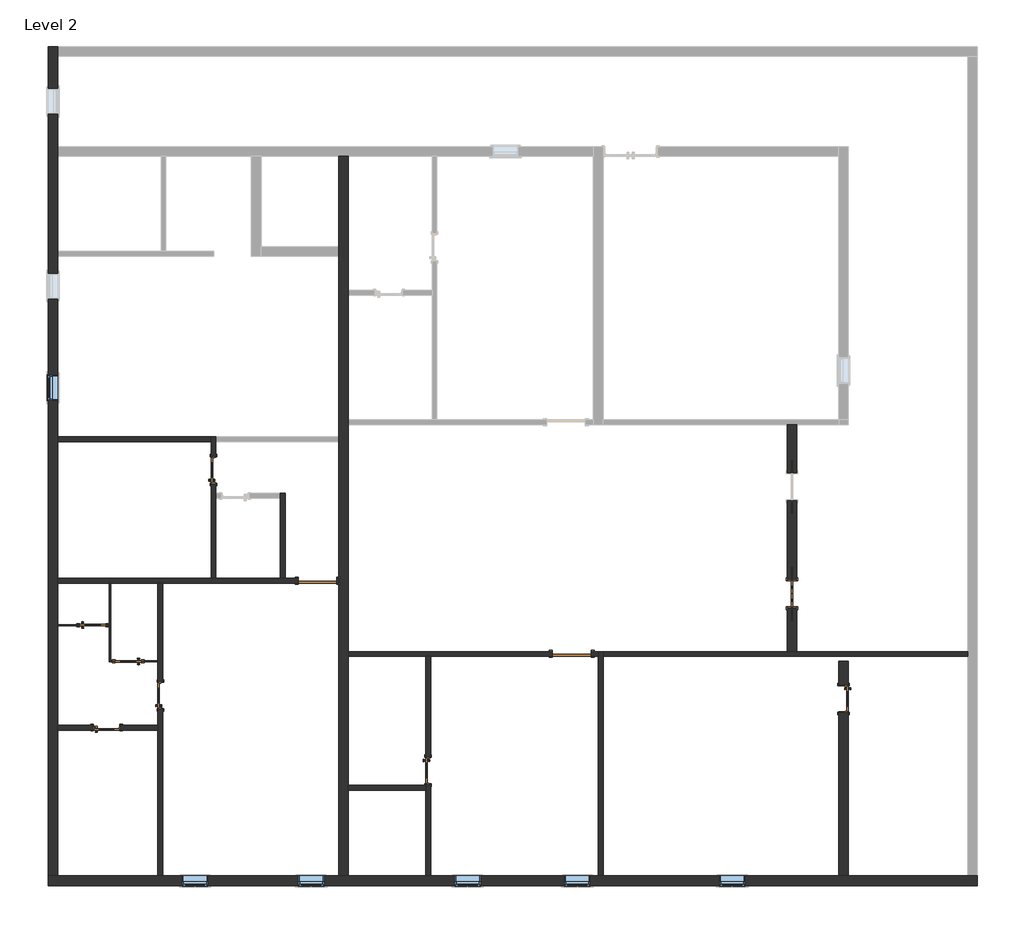
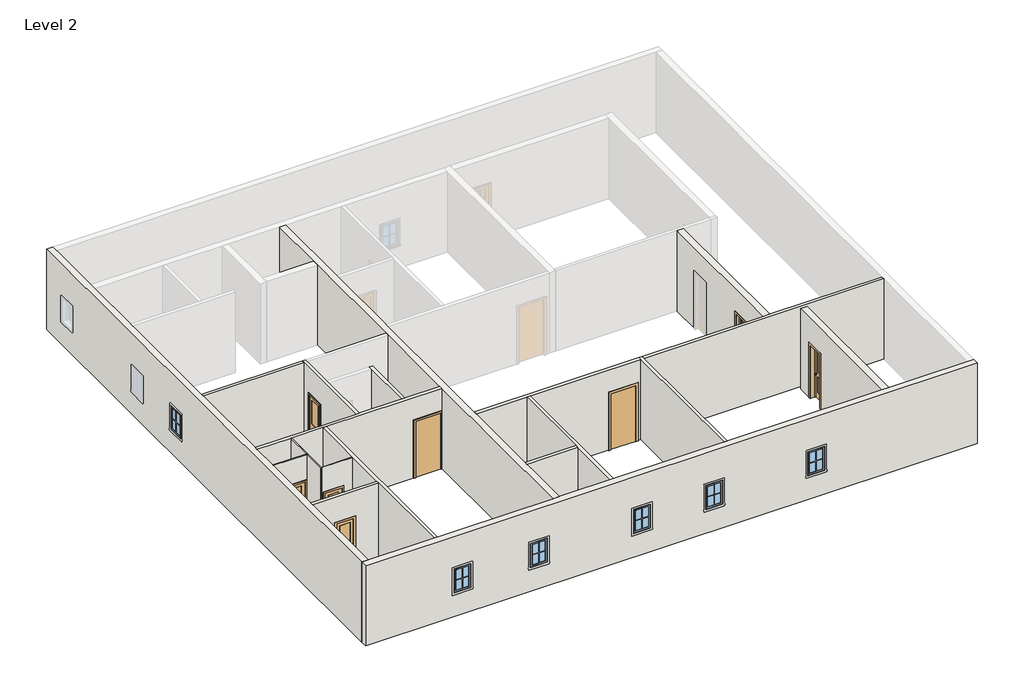
# One storey, part 1 of 2: 19 walls, 10 doors, 6 windows.
"""IFC4 building model written with IfcOpenShell, lengths in millimetres."""

from ifc_helpers import new_model, si_unit, frame, origin, place, context, project, spatial, polyline, outline, extrude, faceted_brep, transform, mapped, element, save
from components import door_interior_double_pocket_2_panel_wood_door_interior_52fbc1e8, door_interior_single_2_panel_wood_door_interior_single_2_03d66c98, door_interior_single_2_panel_wood_door_interior_single_2_a051e6ed, door_interior_single_2_panel_wood_door_interior_single_2_5f4e2ecc, door_interior_single_2_panel_wood_d3_c9a7c184, door_305aa2a5, window_bab9308a, window_25e7c868

model = new_model("IFC4")

# Units and contexts
model_context = context("Model", 3, world=origin())
ifc_project = project(units=[si_unit("LENGTHUNIT", "METRE", prefix="MILLI")], contexts=[model_context])

# Site, building, storey
site = spatial("IfcSite", under=ifc_project)
building = spatial("IfcBuilding", under=site)
storey = spatial("IfcBuildingStorey", under=building, Name="Level 2", Elevation=457.2)

# Doors
placement = place(None, origin())
door_interior_double_pocket_2_panel_wood_door_interior_shape = door_interior_double_pocket_2_panel_wood_door_interior_52fbc1e8(model_context)
element("IfcDoor", 1, ObjectType="Door-Interior-Double-Pocket-2_Panel-Wood : Door-Interior-Double-Pocket-2_Panel-Wood", at=placement, inside=storey, context=model_context, shape_type="MappedRepresentation", body=[
    mapped(door_interior_double_pocket_2_panel_wood_door_interior_shape, transform((5604.2549703, -2194.6409081, 457.2), x_axis=(0.0, -1.0, 0.0), y_axis=(1.0, 0.0, 0.0), z_axis=(0.0, 0.0, 1.0))),
])
door_interior_single_2_panel_wood_door_interior_single_2_shape = door_interior_single_2_panel_wood_door_interior_single_2_03d66c98(model_context)
element("IfcDoor", 2, ObjectType="Door-Interior-Single-2_Panel-Wood : Door-Interior-Single-2_Panel-Wood", at=placement, inside=storey, context=model_context, shape_type="MappedRepresentation", body=[
    mapped(door_interior_single_2_panel_wood_door_interior_single_2_shape, transform((-2989.8496667, -6372.9409081, 457.2), x_axis=(0.0, -1.0, 0.0), y_axis=(1.0, 0.0, 0.0), z_axis=(0.0, 0.0, 1.0))),
])
element("IfcDoor", 3, ObjectType="Door-Interior-Single-2_Panel-Wood : Door-Interior-Single-2_Panel-Wood", at=placement, inside=storey, context=model_context, shape_type="MappedRepresentation", body=[
    mapped(door_interior_single_2_panel_wood_door_interior_single_2_shape, transform((-10578.7200297, -5360.1159081, 457.2), x_axis=(1.0, 0.0, 0.0), y_axis=(0.0, 1.0, 0.0), z_axis=(0.0, 0.0, 1.0))),
])
door_interior_single_2_panel_wood_door_interior_single_2_2_shape = door_interior_single_2_panel_wood_door_interior_single_2_a051e6ed(model_context)
element("IfcDoor", 4, ObjectType="Door-Interior-Single-2_Panel-Wood : Door-Interior-Single-2_Panel-Wood", at=placement, inside=storey, context=model_context, shape_type="MappedRepresentation", body=[
    mapped(door_interior_single_2_panel_wood_door_interior_single_2_2_shape, transform((-9315.0700297, -4594.9409081, 457.2), x_axis=(0.0, 1.0, 0.0), y_axis=(-1.0, 0.0, 0.0), z_axis=(0.0, 0.0, 1.0))),
])
element("IfcDoor", 5, ObjectType="Door-Interior-Single-2_Panel-Wood : Door-Interior-Single-2_Panel-Wood", at=placement, inside=storey, context=model_context, shape_type="MappedRepresentation", body=[
    mapped(door_interior_single_2_panel_wood_door_interior_single_2_2_shape, transform((-8057.7700297, 726.3590919, 457.2), x_axis=(0.0, 1.0, 0.0), y_axis=(-1.0, 0.0, 0.0), z_axis=(0.0, 0.0, 1.0))),
])
door_interior_single_2_panel_wood_door_interior_single_2_3_shape = door_interior_single_2_panel_wood_door_interior_single_2_5f4e2ecc(model_context)
element("IfcDoor", 6, ObjectType="Door-Interior-Single-2_Panel-Wood : Door-Interior-Single-2_Panel-Wood", at=placement, inside=storey, context=model_context, shape_type="MappedRepresentation", body=[
    mapped(door_interior_single_2_panel_wood_door_interior_single_2_3_shape, transform((6826.6299703, -4677.4909081, 457.2), x_axis=(0.0, -1.0, 0.0), y_axis=(1.0, 0.0, 0.0), z_axis=(0.0, 0.0, 1.0))),
])
door_interior_single_2_panel_wood_d3_shape = door_interior_single_2_panel_wood_d3_c9a7c184(model_context)
element("IfcDoor", 7, ObjectType="Door-Interior-Single-2_Panel-Wood : d3", at=placement, inside=storey, context=model_context, shape_type="MappedRepresentation", body=[
    mapped(door_interior_single_2_panel_wood_d3_shape, transform((-10905.7021106, -2941.2913376, 457.2), x_axis=(1.0, 0.0, 0.0), y_axis=(0.0, 1.0, 0.0), z_axis=(0.0, 0.0, 1.0))),
])
element("IfcDoor", 8, ObjectType="Door-Interior-Single-2_Panel-Wood : d3", at=placement, inside=storey, context=model_context, shape_type="MappedRepresentation", body=[
    mapped(door_interior_single_2_panel_wood_d3_shape, transform((-10067.5021106, -3785.3159081, 457.2), x_axis=(-1.0, 0.0, 0.0), y_axis=(0.0, -1.0, 0.0), z_axis=(0.0, 0.0, 1.0))),
])
door_shape = door_305aa2a5(model_context)
element("IfcDoor", 9, ObjectType="Single-Flush : 36\" x 84\"", at=placement, inside=storey, context=model_context, shape_type="MappedRepresentation", body=[
    mapped(door_shape, transform((-5597.1450297, -1889.8409081, 457.2), x_axis=(1.0, 0.0, 0.0), y_axis=(0.0, 1.0, 0.0), z_axis=(0.0, 0.0, 1.0))),
])
element("IfcDoor", 10, ObjectType="Single-Flush : 36\" x 84\"", at=placement, inside=storey, context=model_context, shape_type="MappedRepresentation", body=[
    mapped(door_shape, transform((403.6049703, -3617.0409081, 457.2), x_axis=(1.0, 0.0, 0.0), y_axis=(0.0, 1.0, 0.0), z_axis=(0.0, 0.0, 1.0))),
])

# Walls
element("IfcWall", 11, ObjectType="1\"", at=placement, inside=storey, context=model_context, shape_type="SweptSolid", body=[
    extrude(outline(polyline([(3505.2, -10512.0021106), (3505.2, -11731.2450297), (457.2, -11731.2450297), (457.2, -11235.9021106), (2514.6, -11235.9021106), (2514.6, -10575.5021106), (457.2, -10575.5021106), (457.2, -10512.0021106), (3505.2, -10512.0021106)])), frame((0.0, -2950.8163376, 0.0), z_axis=(0.0, 1.0, 0.0), x_axis=(0.0, 0.0, 1.0)), (0.0, 0.0, 1.0), 25.4),
])
element("IfcWall", 12, ObjectType="1\"", at=placement, inside=storey, context=model_context, shape_type="Brep", body=[
    faceted_brep([(-10486.6021106, -3801.1909081, 457.2), (-10486.6021106, -3775.7909081, 457.2), (-10486.6021106, -1946.9909081, 457.2), (-10486.6021106, -1946.9909081, 3505.2), (-10486.6021106, -3775.7909081, 3505.2), (-10486.6021106, -3801.1909081, 3505.2), (-10512.0021106, -3801.1909081, 457.2), (-10512.0021106, -3801.1909081, 3505.2), (-10512.0021106, -2950.8163376, 3505.2), (-10512.0021106, -2925.4163376, 3505.2), (-10512.0021106, -1946.9909081, 3505.2), (-10512.0021106, -1946.9909081, 457.2), (-10512.0021106, -2925.4163376, 457.2), (-10512.0021106, -2950.8163376, 457.2)], [[[0, 1, 2, 3, 4, 5]], [[6, 7, 8, 9, 10, 11, 12, 13]], [[2, 1, 0, 6, 13, 12, 11]], [[5, 4, 3, 10, 9, 8, 7]], [[3, 2, 11, 10]], [[0, 5, 7, 6]]]),
])
element("IfcWall", 13, ObjectType="1\"", at=placement, inside=storey, context=model_context, shape_type="SweptSolid", body=[
    extrude(outline(polyline([(3505.2, -9369.0450297), (3505.2, -10486.6021106), (457.2, -10486.6021106), (457.2, -10397.7021106), (2514.6, -10397.7021106), (2514.6, -9737.3021106), (457.2, -9737.3021106), (457.2, -9369.0450297), (3505.2, -9369.0450297)])), frame((0.0, -3801.1909081, 0.0), z_axis=(0.0, 1.0, 0.0), x_axis=(0.0, 0.0, 1.0)), (0.0, 0.0, 1.0), 25.4),
])
element("IfcWall", 14, ObjectType="4.5\" wall", at=placement, inside=storey, context=model_context, shape_type="Brep", body=[
    faceted_brep([(-9254.7450297, -1946.9909081, 3505.2), (-9254.7450297, -8855.7909081, 3505.2), (-9254.7450297, -8855.7909081, 457.2), (-9254.7450297, -4925.1409081, 457.2), (-9254.7450297, -4925.1409081, 2514.6), (-9254.7450297, -4264.7409081, 2514.6), (-9254.7450297, -4264.7409081, 457.2), (-9254.7450297, -1946.9909081, 457.2), (-9369.0450297, -8855.7909081, 3505.2), (-9369.0450297, -5414.0909081, 3505.2), (-9369.0450297, -5299.7909081, 3505.2), (-9369.0450297, -3801.1909081, 3505.2), (-9369.0450297, -3775.7909081, 3505.2), (-9369.0450297, -1946.9909081, 3505.2), (-9369.0450297, -1946.9909081, 457.2), (-9369.0450297, -3775.7909081, 457.2), (-9369.0450297, -3801.1909081, 457.2), (-9369.0450297, -4264.7409081, 457.2), (-9369.0450297, -4264.7409081, 2514.6), (-9369.0450297, -4925.1409081, 2514.6), (-9369.0450297, -4925.1409081, 457.2), (-9369.0450297, -5299.7909081, 457.2), (-9369.0450297, -5414.0909081, 457.2), (-9369.0450297, -8855.7909081, 457.2)], [[[0, 1, 2, 3, 4, 5, 6, 7]], [[8, 9, 10, 11, 12, 13, 14, 15, 16, 17, 18, 19, 20, 21, 22, 23]], [[2, 23, 22, 21, 20, 3]], [[14, 7, 6, 17, 16, 15]], [[1, 0, 13, 12, 11, 10, 9, 8]], [[2, 1, 8, 23]], [[0, 7, 14, 13]], [[5, 18, 17, 6]], [[18, 5, 4, 19]], [[19, 4, 3, 20]]]),
])
element("IfcWall", 15, ObjectType="4.5\" wall", at=placement, inside=storey, context=model_context, shape_type="SweptSolid", body=[
    extrude(outline(polyline([(3505.2, -9369.0450297), (3505.2, -11731.2450297), (457.2, -11731.2450297), (457.2, -10908.9200297), (2514.6, -10908.9200297), (2514.6, -10248.5200297), (457.2, -10248.5200297), (457.2, -9369.0450297), (3505.2, -9369.0450297)])), frame((0.0, -5414.0909081, 0.0), z_axis=(0.0, 1.0, 0.0), x_axis=(0.0, 0.0, 1.0)), (0.0, 0.0, 1.0), 114.3),
])
element("IfcWall", 16, ObjectType="4.5\" wall", at=placement, inside=storey, context=model_context, shape_type="Brep", body=[
    faceted_brep([(-5139.9450297, -1946.9909081, 2590.8), (-5139.9450297, -1946.9909081, 457.2), (-5101.8450297, -1946.9909081, 457.2), (-5101.8450297, -1946.9909081, 3505.2), (-9254.7450297, -1946.9909081, 3505.2), (-9369.0450297, -1946.9909081, 3505.2), (-10486.6021106, -1946.9909081, 3505.2), (-10512.0021106, -1946.9909081, 3505.2), (-11731.2450297, -1946.9909081, 3505.2), (-11731.2450297, -1946.9909081, 457.2), (-10512.0021106, -1946.9909081, 457.2), (-10486.6021106, -1946.9909081, 457.2), (-9369.0450297, -1946.9909081, 457.2), (-9254.7450297, -1946.9909081, 457.2), (-6054.3450297, -1946.9909081, 457.2), (-6054.3450297, -1946.9909081, 2590.8), (-5101.8450297, -1832.6909081, 457.2), (-5139.9450297, -1832.6909081, 457.2), (-5139.9450297, -1832.6909081, 2590.8), (-6054.3450297, -1832.6909081, 2590.8), (-6054.3450297, -1832.6909081, 457.2), (-6359.1450297, -1832.6909081, 457.2), (-6473.4450297, -1832.6909081, 457.2), (-7997.4450297, -1832.6909081, 457.2), (-8111.7450297, -1832.6909081, 457.2), (-11731.2450297, -1832.6909081, 457.2), (-11731.2450297, -1832.6909081, 3505.2), (-8111.7450297, -1832.6909081, 3505.2), (-7997.4450297, -1832.6909081, 3505.2), (-6473.4450297, -1832.6909081, 3505.2), (-6359.1450297, -1832.6909081, 3505.2), (-5101.8450297, -1832.6909081, 3505.2)], [[[0, 1, 2, 3, 4, 5, 6, 7, 8, 9, 10, 11, 12, 13, 14, 15]], [[16, 17, 18, 19, 20, 21, 22, 23, 24, 25, 26, 27, 28, 29, 30, 31]], [[2, 1, 17, 16]], [[14, 13, 12, 11, 10, 9, 25, 24, 23, 22, 21, 20]], [[8, 7, 6, 5, 4, 3, 31, 30, 29, 28, 27, 26]], [[9, 8, 26, 25]], [[3, 2, 16, 31]], [[18, 17, 1, 0]], [[19, 18, 0, 15]], [[20, 19, 15, 14]]]),
])
element("IfcWall", 17, ObjectType="4.5\" wall", at=placement, inside=storey, context=model_context, shape_type="Brep", body=[
    faceted_brep([(-6359.1450297, -1832.6909081, 457.2), (-6359.1450297, 173.9090919, 457.2), (-6359.1450297, 173.9090919, 3505.2), (-6359.1450297, -1832.6909081, 3505.2), (-6473.4450297, -1832.6909081, 457.2), (-6473.4450297, -1832.6909081, 3505.2), (-6473.4450297, 59.6090919, 3505.2), (-6473.4450297, 173.9090919, 3505.2), (-6473.4450297, 173.9090919, 457.2), (-6473.4450297, 59.6090919, 457.2)], [[[0, 1, 2, 3]], [[4, 5, 6, 7, 8, 9]], [[1, 0, 4, 9, 8]], [[3, 2, 7, 6, 5]], [[0, 3, 5, 4]], [[2, 1, 8, 7]]]),
])
element("IfcWall", 18, ObjectType="4.5\" wall", at=placement, inside=storey, context=model_context, shape_type="Brep", body=[
    faceted_brep([(-8111.7450297, -1832.6909081, 3505.2), (-8111.7450297, 1393.1090919, 3505.2), (-8111.7450297, 1507.4090919, 3505.2), (-8111.7450297, 1507.4090919, 457.2), (-8111.7450297, 1393.1090919, 457.2), (-8111.7450297, 1056.5590919, 457.2), (-8111.7450297, 1056.5590919, 2514.6), (-8111.7450297, 396.1590919, 2514.6), (-8111.7450297, 396.1590919, 457.2), (-8111.7450297, -1832.6909081, 457.2), (-7997.4450297, 1507.4090919, 3505.2), (-7997.4450297, 1393.1090919, 3505.2), (-7997.4450297, 173.9090919, 3505.2), (-7997.4450297, 59.6090919, 3505.2), (-7997.4450297, -1832.6909081, 3505.2), (-7997.4450297, -1832.6909081, 457.2), (-7997.4450297, 59.6090919, 457.2), (-7997.4450297, 173.9090919, 457.2), (-7997.4450297, 396.1590919, 457.2), (-7997.4450297, 396.1590919, 2514.6), (-7997.4450297, 1056.5590919, 2514.6), (-7997.4450297, 1056.5590919, 457.2), (-7997.4450297, 1393.1090919, 457.2), (-7997.4450297, 1507.4090919, 457.2)], [[[0, 1, 2, 3, 4, 5, 6, 7, 8, 9]], [[10, 11, 12, 13, 14, 15, 16, 17, 18, 19, 20, 21, 22, 23]], [[15, 9, 8, 18, 17, 16]], [[3, 23, 22, 21, 5, 4]], [[2, 1, 0, 14, 13, 12, 11, 10]], [[0, 9, 15, 14]], [[3, 2, 10, 23]], [[20, 6, 5, 21]], [[6, 20, 19, 7]], [[7, 19, 18, 8]]]),
])
element("IfcWall", 19, ObjectType="4.5\" wall", at=placement, inside=storey, context=model_context, shape_type="SweptSolid", body=[
    extrude(outline(polyline([(-8111.7450297, 1393.1090919), (-11731.2450297, 1393.1090919), (-11731.2450297, 1507.4090919), (-8111.7450297, 1507.4090919), (-8111.7450297, 1393.1090919)])), frame((0.0, 0.0, 457.2), z_axis=(0.0, 0.0, 1.0), x_axis=(1.0, 0.0, 0.0)), (0.0, 0.0, 1.0), 3048.0),
])
element("IfcWall", 20, ObjectType="4.5\" wall", at=placement, inside=storey, context=model_context, shape_type="Brep", body=[
    faceted_brep([(1146.5549703, -8855.7909081, 457.2), (1146.5549703, -3674.1909081, 457.2), (1146.5549703, -3559.8909081, 457.2), (1146.5549703, -3559.8909081, 3505.2), (1146.5549703, -3674.1909081, 3505.2), (1146.5549703, -8855.7909081, 3505.2), (1032.2549703, -8855.7909081, 457.2), (1032.2549703, -8855.7909081, 3505.2), (1032.2549703, -3674.1909081, 3505.2), (1032.2549703, -3559.8909081, 3505.2), (1032.2549703, -3559.8909081, 457.2), (1032.2549703, -3674.1909081, 457.2)], [[[0, 1, 2, 3, 4, 5]], [[6, 7, 8, 9, 10, 11]], [[2, 1, 0, 6, 11, 10]], [[5, 4, 3, 9, 8, 7]], [[0, 5, 7, 6]], [[3, 2, 10, 9]]]),
])
element("IfcWall", 21, ObjectType="4.5\" wall", at=placement, inside=storey, context=model_context, shape_type="Brep", body=[
    faceted_brep([(1146.5549703, -3674.1909081, 457.2), (9757.1549703, -3674.1909081, 457.2), (9757.1549703, -3674.1909081, 3505.2), (1146.5549703, -3674.1909081, 3505.2), (1146.5549703, -3559.8909081, 457.2), (1146.5549703, -3559.8909081, 3505.2), (5489.9549703, -3559.8909081, 3505.2), (5718.5549703, -3559.8909081, 3505.2), (9757.1549703, -3559.8909081, 3505.2), (9757.1549703, -3559.8909081, 457.2), (5718.5549703, -3559.8909081, 457.2), (5489.9549703, -3559.8909081, 457.2)], [[[0, 1, 2, 3]], [[4, 5, 6, 7, 8, 9, 10, 11]], [[1, 0, 4, 11, 10, 9]], [[3, 2, 8, 7, 6, 5]], [[0, 3, 5, 4]], [[2, 1, 9, 8]]]),
])
element("IfcWall", 22, ObjectType="4.5\" wall", at=placement, inside=storey, context=model_context, shape_type="Brep", body=[
    faceted_brep([(860.8049703, -3674.1909081, 2590.8), (860.8049703, -3674.1909081, 457.2), (1032.2549703, -3674.1909081, 457.2), (1032.2549703, -3674.1909081, 3505.2), (-2929.5246667, -3674.1909081, 3505.2), (-3043.8246667, -3674.1909081, 3505.2), (-4872.6246667, -3674.1909081, 3505.2), (-4872.6246667, -3674.1909081, 457.2), (-3043.8246667, -3674.1909081, 457.2), (-2929.5246667, -3674.1909081, 457.2), (-53.5950297, -3674.1909081, 457.2), (-53.5950297, -3674.1909081, 2590.8), (1032.2549703, -3559.8909081, 457.2), (860.8049703, -3559.8909081, 457.2), (860.8049703, -3559.8909081, 2590.8), (-53.5950297, -3559.8909081, 2590.8), (-53.5950297, -3559.8909081, 457.2), (-4872.6246667, -3559.8909081, 457.2), (-4872.6246667, -3559.8909081, 3505.2), (1032.2549703, -3559.8909081, 3505.2)], [[[0, 1, 2, 3, 4, 5, 6, 7, 8, 9, 10, 11]], [[12, 13, 14, 15, 16, 17, 18, 19]], [[2, 1, 13, 12]], [[10, 9, 8, 7, 17, 16]], [[6, 5, 4, 3, 19, 18]], [[7, 6, 18, 17]], [[3, 2, 12, 19]], [[14, 13, 1, 0]], [[15, 14, 0, 11]], [[16, 15, 11, 10]]]),
])
element("IfcWall", 23, ObjectType="4.5\" wall", at=placement, inside=storey, context=model_context, shape_type="SweptSolid", body=[
    extrude(outline(polyline([(-3043.8246667, -6836.4909081), (-4872.6246667, -6836.4909081), (-4872.6246667, -6722.1909081), (-3043.8246667, -6722.1909081), (-3043.8246667, -6836.4909081)])), frame((0.0, 0.0, 457.2), z_axis=(0.0, 0.0, 1.0), x_axis=(1.0, 0.0, 0.0)), (0.0, 0.0, 1.0), 3048.0),
])
element("IfcWall", 24, ObjectType="4.5\" wall", at=placement, inside=storey, context=model_context, shape_type="Brep", body=[
    faceted_brep([(-2929.5246667, -3674.1909081, 3505.2), (-2929.5246667, -8855.7909081, 3505.2), (-2929.5246667, -8855.7909081, 457.2), (-2929.5246667, -6703.1409081, 457.2), (-2929.5246667, -6703.1409081, 2514.6), (-2929.5246667, -6042.7409081, 2514.6), (-2929.5246667, -6042.7409081, 457.2), (-2929.5246667, -3674.1909081, 457.2), (-3043.8246667, -8855.7909081, 3505.2), (-3043.8246667, -6836.4909081, 3505.2), (-3043.8246667, -6722.1909081, 3505.2), (-3043.8246667, -3674.1909081, 3505.2), (-3043.8246667, -3674.1909081, 457.2), (-3043.8246667, -6042.7409081, 457.2), (-3043.8246667, -6042.7409081, 2514.6), (-3043.8246667, -6703.1409081, 2514.6), (-3043.8246667, -6703.1409081, 457.2), (-3043.8246667, -6722.1909081, 457.2), (-3043.8246667, -6836.4909081, 457.2), (-3043.8246667, -8855.7909081, 457.2)], [[[0, 1, 2, 3, 4, 5, 6, 7]], [[8, 9, 10, 11, 12, 13, 14, 15, 16, 17, 18, 19]], [[2, 19, 18, 17, 16, 3]], [[12, 7, 6, 13]], [[1, 0, 11, 10, 9, 8]], [[2, 1, 8, 19]], [[0, 7, 12, 11]], [[15, 4, 3, 16]], [[4, 15, 14, 5]], [[5, 14, 13, 6]]]),
])
element("IfcWall", 25, ObjectType="9\" wall", at=placement, inside=storey, context=model_context, shape_type="Brep", body=[
    faceted_brep([(-11959.8450297, -9085.9784081, 457.2), (9985.7549703, -9085.9784081, 457.2), (9985.7549703, -9085.9784081, 3505.2), (-11959.8450297, -9085.9784081, 3505.2), (4499.3549703, -9085.9784081, 2286.0), (4499.3549703, -9085.9784081, 1371.6), (3889.7549703, -9085.9784081, 1371.6), (3889.7549703, -9085.9784081, 2286.0), (232.1549703, -9085.9784081, 2286.0), (841.7549703, -9085.9784081, 2286.0), (841.7549703, -9085.9784081, 1371.6), (232.1549703, -9085.9784081, 1371.6), (-2358.6450297, -9085.9784081, 2286.0), (-1749.0450297, -9085.9784081, 2286.0), (-1749.0450297, -9085.9784081, 1371.6), (-2358.6450297, -9085.9784081, 1371.6), (-6054.3450297, -9085.9784081, 2286.0), (-5444.7450297, -9085.9784081, 2286.0), (-5444.7450297, -9085.9784081, 1371.6), (-6054.3450297, -9085.9784081, 1371.6), (-8797.5450297, -9085.9784081, 2286.0), (-8187.9450297, -9085.9784081, 2286.0), (-8187.9450297, -9085.9784081, 1371.6), (-8797.5450297, -9085.9784081, 1371.6), (-11959.8450297, -8857.3784081, 457.2), (-11959.8450297, -8857.3784081, 3505.2), (-11731.2450297, -8857.3784081, 3505.2), (-5101.8450297, -8857.3784081, 3505.2), (-4873.2450297, -8857.3784081, 3505.2), (9985.7549703, -8857.3784081, 3505.2), (9985.7549703, -8857.3784081, 457.2), (-4873.2450297, -8857.3784081, 457.2), (-5101.8450297, -8857.3784081, 457.2), (-11731.2450297, -8857.3784081, 457.2), (4499.3549703, -8857.3784081, 2286.0), (3889.7549703, -8857.3784081, 2286.0), (3889.7549703, -8857.3784081, 1371.6), (4499.3549703, -8857.3784081, 1371.6), (232.1549703, -8857.3784081, 2286.0), (232.1549703, -8857.3784081, 1371.6), (841.7549703, -8857.3784081, 1371.6), (841.7549703, -8857.3784081, 2286.0), (-2358.6450297, -8857.3784081, 2286.0), (-2358.6450297, -8857.3784081, 1371.6), (-1749.0450297, -8857.3784081, 1371.6), (-1749.0450297, -8857.3784081, 2286.0), (-6054.3450297, -8857.3784081, 2286.0), (-6054.3450297, -8857.3784081, 1371.6), (-5444.7450297, -8857.3784081, 1371.6), (-5444.7450297, -8857.3784081, 2286.0), (-8797.5450297, -8857.3784081, 2286.0), (-8797.5450297, -8857.3784081, 1371.6), (-8187.9450297, -8857.3784081, 1371.6), (-8187.9450297, -8857.3784081, 2286.0)], [[[0, 1, 2, 3], [4, 5, 6, 7], [8, 9, 10, 11], [12, 13, 14, 15], [16, 17, 18, 19], [20, 21, 22, 23]], [[24, 25, 26, 27, 28, 29, 30, 31, 32, 33], [34, 35, 36, 37], [38, 39, 40, 41], [42, 43, 44, 45], [46, 47, 48, 49], [50, 51, 52, 53]], [[1, 0, 24, 33, 32, 31, 30]], [[2, 1, 30, 29]], [[3, 2, 29, 28, 27, 26, 25]], [[0, 3, 25, 24]], [[5, 4, 34, 37]], [[6, 5, 37, 36]], [[7, 6, 36, 35]], [[4, 7, 35, 34]], [[39, 38, 8, 11]], [[40, 39, 11, 10]], [[41, 40, 10, 9]], [[38, 41, 9, 8]], [[43, 42, 12, 15]], [[44, 43, 15, 14]], [[45, 44, 14, 13]], [[42, 45, 13, 12]], [[47, 46, 16, 19]], [[48, 47, 19, 18]], [[49, 48, 18, 17]], [[46, 49, 17, 16]], [[51, 50, 20, 23]], [[52, 51, 23, 22]], [[53, 52, 22, 21]], [[50, 53, 21, 20]]]),
])
element("IfcWall", 26, ObjectType="9\" wall", at=placement, inside=storey, context=model_context, shape_type="Brep", body=[
    faceted_brep([(-11959.8450297, 10727.6090919, 457.2), (-11959.8450297, -8857.3784081, 457.2), (-11959.8450297, -8857.3784081, 3505.2), (-11959.8450297, 10727.6090919, 3505.2), (-11959.8450297, 9127.4090919, 2286.0), (-11959.8450297, 9127.4090919, 1371.6), (-11959.8450297, 9737.0090919, 1371.6), (-11959.8450297, 9737.0090919, 2286.0), (-11959.8450297, 5374.5590919, 2286.0), (-11959.8450297, 4764.9590919, 2286.0), (-11959.8450297, 4764.9590919, 1371.6), (-11959.8450297, 5374.5590919, 1371.6), (-11959.8450297, 2974.2590919, 2286.0), (-11959.8450297, 2364.6590919, 2286.0), (-11959.8450297, 2364.6590919, 1371.6), (-11959.8450297, 2974.2590919, 1371.6), (-11731.2450297, 10727.6090919, 457.2), (-11731.2450297, 10727.6090919, 3505.2), (-11731.2450297, 10499.0090919, 3505.2), (-11731.2450297, 8365.4090919, 3505.2), (-11731.2450297, 8136.8090919, 3505.2), (-11731.2450297, 5888.9090919, 3505.2), (-11731.2450297, 5774.6090919, 3505.2), (-11731.2450297, 1507.4090919, 3505.2), (-11731.2450297, 1393.1090919, 3505.2), (-11731.2450297, -1832.6909081, 3505.2), (-11731.2450297, -1946.9909081, 3505.2), (-11731.2450297, -2925.4163376, 3505.2), (-11731.2450297, -2950.8163376, 3505.2), (-11731.2450297, -5299.7909081, 3505.2), (-11731.2450297, -5414.0909081, 3505.2), (-11731.2450297, -8857.3784081, 3505.2), (-11731.2450297, -8857.3784081, 457.2), (-11731.2450297, -5414.0909081, 457.2), (-11731.2450297, -5299.7909081, 457.2), (-11731.2450297, -2950.8163376, 457.2), (-11731.2450297, -2925.4163376, 457.2), (-11731.2450297, -1946.9909081, 457.2), (-11731.2450297, -1832.6909081, 457.2), (-11731.2450297, 1393.1090919, 457.2), (-11731.2450297, 1507.4090919, 457.2), (-11731.2450297, 5774.6090919, 457.2), (-11731.2450297, 5888.9090919, 457.2), (-11731.2450297, 8136.8090919, 457.2), (-11731.2450297, 8365.4090919, 457.2), (-11731.2450297, 10499.0090919, 457.2), (-11731.2450297, 9127.4090919, 2286.0), (-11731.2450297, 9737.0090919, 2286.0), (-11731.2450297, 9737.0090919, 1371.6), (-11731.2450297, 9127.4090919, 1371.6), (-11731.2450297, 5374.5590919, 2286.0), (-11731.2450297, 5374.5590919, 1371.6), (-11731.2450297, 4764.9590919, 1371.6), (-11731.2450297, 4764.9590919, 2286.0), (-11731.2450297, 2974.2590919, 2286.0), (-11731.2450297, 2974.2590919, 1371.6), (-11731.2450297, 2364.6590919, 1371.6), (-11731.2450297, 2364.6590919, 2286.0)], [[[0, 1, 2, 3], [4, 5, 6, 7], [8, 9, 10, 11], [12, 13, 14, 15]], [[16, 17, 18, 19, 20, 21, 22, 23, 24, 25, 26, 27, 28, 29, 30, 31, 32, 33, 34, 35, 36, 37, 38, 39, 40, 41, 42, 43, 44, 45], [46, 47, 48, 49], [50, 51, 52, 53], [54, 55, 56, 57]], [[1, 0, 16, 45, 44, 43, 42, 41, 40, 39, 38, 37, 36, 35, 34, 33, 32]], [[3, 2, 31, 30, 29, 28, 27, 26, 25, 24, 23, 22, 21, 20, 19, 18, 17]], [[2, 1, 32, 31]], [[5, 4, 46, 49]], [[6, 5, 49, 48]], [[7, 6, 48, 47]], [[4, 7, 47, 46]], [[51, 50, 8, 11]], [[52, 51, 11, 10]], [[53, 52, 10, 9]], [[50, 53, 9, 8]], [[55, 54, 12, 15]], [[56, 55, 15, 14]], [[57, 56, 14, 13]], [[54, 57, 13, 12]], [[0, 3, 17, 16]]]),
])
element("IfcWall", 27, ObjectType="9\" wall", at=placement, inside=storey, context=model_context, shape_type="Brep", body=[
    faceted_brep([(-5101.8450297, 8136.8090919, 457.2), (-5101.8450297, 6003.2090919, 457.2), (-5101.8450297, 5774.6090919, 457.2), (-5101.8450297, 1507.4090919, 457.2), (-5101.8450297, 1393.1090919, 457.2), (-5101.8450297, -1832.6909081, 457.2), (-5101.8450297, -1946.9909081, 457.2), (-5101.8450297, -8857.3784081, 457.2), (-5101.8450297, -8857.3784081, 3505.2), (-5101.8450297, -1946.9909081, 3505.2), (-5101.8450297, -1832.6909081, 3505.2), (-5101.8450297, 1393.1090919, 3505.2), (-5101.8450297, 1507.4090919, 3505.2), (-5101.8450297, 5774.6090919, 3505.2), (-5101.8450297, 6003.2090919, 3505.2), (-5101.8450297, 8136.8090919, 3505.2), (-4873.2450297, 8136.8090919, 457.2), (-4873.2450297, 8136.8090919, 3505.2), (-4873.2450297, 4974.5090919, 3505.2), (-4873.2450297, 4860.2090919, 3505.2), (-4873.2450297, 1913.8090919, 3505.2), (-4873.2450297, 1799.5090919, 3505.2), (-4873.2450297, -8857.3784081, 3505.2), (-4873.2450297, -8857.3784081, 457.2), (-4873.2450297, 1799.5090919, 457.2), (-4873.2450297, 1913.8090919, 457.2), (-4873.2450297, 4860.2090919, 457.2), (-4873.2450297, 4974.5090919, 457.2)], [[[0, 1, 2, 3, 4, 5, 6, 7, 8, 9, 10, 11, 12, 13, 14, 15]], [[16, 17, 18, 19, 20, 21, 22, 23, 24, 25, 26, 27]], [[7, 6, 5, 4, 3, 2, 1, 0, 16, 27, 26, 25, 24, 23]], [[15, 14, 13, 12, 11, 10, 9, 8, 22, 21, 20, 19, 18, 17]], [[0, 15, 17, 16]], [[8, 7, 23, 22]]]),
])
element("IfcWall", 28, ObjectType="9\" wall", at=placement, inside=storey, context=model_context, shape_type="SweptSolid", body=[
    extrude(outline(polyline([(-3788.4909081, 3505.2), (-3788.4909081, 457.2), (-4347.2909081, 457.2), (-4347.2909081, 2514.6), (-5007.6909081, 2514.6), (-5007.6909081, 457.2), (-8855.7909081, 457.2), (-8855.7909081, 3505.2), (-3788.4909081, 3505.2)])), frame((6709.1549703, 0.0, 0.0), z_axis=(1.0, 0.0, 0.0), x_axis=(0.0, 1.0, 0.0)), (0.0, 0.0, 1.0), 228.6),
])
element("IfcWall", 29, ObjectType="9\" wall", at=placement, inside=storey, context=model_context, shape_type="Brep", body=[
    faceted_brep([(5718.5549703, 1799.5090919, 3505.2), (5718.5549703, -3559.8909081, 3505.2), (5718.5549703, -3559.8909081, 457.2), (5718.5549703, -2524.8409081, 457.2), (5718.5549703, -2524.8409081, 2616.2), (5718.5549703, -1864.4409081, 2616.2), (5718.5549703, -1864.4409081, 457.2), (5718.5549703, 2.4590919, 457.2), (5718.5549703, 2.4590919, 2616.2), (5718.5549703, 662.8590919, 2616.2), (5718.5549703, 662.8590919, 457.2), (5718.5549703, 1799.5090919, 457.2), (5489.9549703, -3559.8909081, 3505.2), (5489.9549703, 1799.5090919, 3505.2), (5489.9549703, 1799.5090919, 457.2), (5489.9549703, 662.8590919, 457.2), (5489.9549703, 662.8590919, 2616.2), (5489.9549703, 2.4590919, 2616.2), (5489.9549703, 2.4590919, 457.2), (5489.9549703, -1864.4409081, 457.2), (5489.9549703, -1864.4409081, 2616.2), (5489.9549703, -2524.8409081, 2616.2), (5489.9549703, -2524.8409081, 457.2), (5489.9549703, -3559.8909081, 457.2), (5583.6174703, -2524.8409081, 457.2), (5583.6174703, -2829.6409081, 457.2), (5624.8924703, -2829.6409081, 457.2), (5624.8924703, -2524.8409081, 457.2), (5624.8924703, 662.8590919, 457.2), (5624.8924703, 967.6590919, 457.2), (5583.6174703, 967.6590919, 457.2), (5583.6174703, 662.8590919, 457.2), (5624.8924703, -302.3409081, 457.2), (5624.8924703, 2.4590919, 457.2), (5624.8924703, -1864.4409081, 457.2), (5624.8924703, -1559.6409081, 457.2), (5583.6174703, -1559.6409081, 457.2), (5583.6174703, -1864.4409081, 457.2), (5583.6174703, 2.4590919, 457.2), (5583.6174703, -302.3409081, 457.2), (5624.8924703, -302.3409081, 2616.2), (5583.6174703, -302.3409081, 2616.2), (5583.6174703, 2.4590919, 2616.2), (5583.6174703, 662.8590919, 2616.2), (5583.6174703, 967.6590919, 2616.2), (5624.8924703, 967.6590919, 2616.2), (5624.8924703, 662.8590919, 2616.2), (5624.8924703, 2.4590919, 2616.2), (5624.8924703, -2829.6409081, 2616.2), (5583.6174703, -2829.6409081, 2616.2), (5583.6174703, -2524.8409081, 2616.2), (5583.6174703, -1864.4409081, 2616.2), (5583.6174703, -1559.6409081, 2616.2), (5624.8924703, -1559.6409081, 2616.2), (5624.8924703, -1864.4409081, 2616.2), (5624.8924703, -2524.8409081, 2616.2)], [[[0, 1, 2, 3, 4, 5, 6, 7, 8, 9, 10, 11]], [[12, 13, 14, 15, 16, 17, 18, 19, 20, 21, 22, 23]], [[2, 23, 22, 24, 25, 26, 27, 3]], [[14, 11, 10, 28, 29, 30, 31, 15]], [[32, 33, 7, 6, 34, 35, 36, 37, 19, 18, 38, 39]], [[1, 0, 13, 12]], [[2, 1, 12, 23]], [[0, 11, 14, 13]], [[40, 41, 42, 17, 16, 43, 44, 45, 46, 9, 8, 47]], [[40, 47, 33, 32]], [[47, 8, 7, 33]], [[9, 46, 28, 10]], [[46, 45, 29, 28]], [[45, 44, 30, 29]], [[44, 43, 31, 30]], [[43, 16, 15, 31]], [[17, 42, 38, 18]], [[42, 41, 39, 38]], [[41, 40, 32, 39]], [[48, 49, 50, 21, 20, 51, 52, 53, 54, 5, 4, 55]], [[48, 55, 27, 26]], [[55, 4, 3, 27]], [[5, 54, 34, 6]], [[54, 53, 35, 34]], [[53, 52, 36, 35]], [[52, 51, 37, 36]], [[51, 20, 19, 37]], [[21, 50, 24, 22]], [[50, 49, 25, 24]], [[49, 48, 26, 25]]]),
])

# Windows
window_shape = window_bab9308a(model_context)
element("IfcWindow", 30, ObjectType="Window-Casement-Single_Left : 24\" x 36\"", at=placement, inside=storey, context=model_context, shape_type="MappedRepresentation", body=[
    mapped(window_shape, transform((536.9549703, -8971.6784081, 457.2), x_axis=(-1.0, 0.0, 0.0), y_axis=(0.0, -1.0, 0.0), z_axis=(0.0, 0.0, 1.0))),
])
element("IfcWindow", 31, ObjectType="Window-Casement-Single_Left : 24\" x 36\"", at=placement, inside=storey, context=model_context, shape_type="MappedRepresentation", body=[
    mapped(window_shape, transform((-2053.8450297, -8971.6784081, 457.2), x_axis=(-1.0, 0.0, 0.0), y_axis=(0.0, -1.0, 0.0), z_axis=(0.0, 0.0, 1.0))),
])
element("IfcWindow", 32, ObjectType="Window-Casement-Single_Left : 24\" x 36\"", at=placement, inside=storey, context=model_context, shape_type="MappedRepresentation", body=[
    mapped(window_shape, transform((-5749.5450297, -8971.6784081, 457.2), x_axis=(-1.0, 0.0, 0.0), y_axis=(0.0, -1.0, 0.0), z_axis=(0.0, 0.0, 1.0))),
])
element("IfcWindow", 33, ObjectType="Window-Casement-Single_Left : 24\" x 36\"", at=placement, inside=storey, context=model_context, shape_type="MappedRepresentation", body=[
    mapped(window_shape, transform((-8492.7450297, -8971.6784081, 457.2), x_axis=(-1.0, 0.0, 0.0), y_axis=(0.0, -1.0, 0.0), z_axis=(0.0, 0.0, 1.0))),
])
element("IfcWindow", 34, ObjectType="Window-Casement-Single_Left : 24\" x 36\"", at=placement, inside=storey, context=model_context, shape_type="MappedRepresentation", body=[
    mapped(window_shape, transform((-11845.5450297, 2669.4590919, 457.2), x_axis=(0.0, 1.0, 0.0), y_axis=(-1.0, 0.0, 0.0), z_axis=(0.0, 0.0, 1.0))),
])
window_2_shape = window_25e7c868(model_context)
element("IfcWindow", 35, ObjectType="Window-Casement-Single_Left : 24\" x 36\"", at=placement, inside=storey, context=model_context, shape_type="MappedRepresentation", body=[
    mapped(window_2_shape, transform((4194.5549703, -8971.6784081, 457.2), x_axis=(1.0, 0.0, 0.0), y_axis=(0.0, 1.0, 0.0), z_axis=(0.0, 0.0, 1.0))),
])

save(model, "model.ifc")

# Revit data of these elements
# Type "Door-Interior-Double-Pocket-2_Panel-Wood : Door-Interior-Double-Pocket-2_Panel-Wood"
#   Type Mark = "14"
#   Assembly Code = "C1020300"
#   Analytic Construction = "Wooden"
#   Top Rail = 0' - 4 11/16"
#   Thickness = 0' - 1 3/8"
#   Thermal Resistance (R) = 2.5876 (h·ft²·°F)/BTU
#   Stiles = 0' - 4 3/4"
#   Rough Width = 4' - 2"
#   Rough Height = 7' - 4 1/2"
#   Panel Width = 1' - 0"
#   Lock Rail = 0' - 7 1/2"
#   Location [instance default] = 1' - 1"
#   Height = 7' - 0"
#   Width = 2' - 0"
#   Heat Transfer Coefficient (U) = 0.3865 BTU/(h·ft²·°F)
#   Bottom Rail = 0' - 9 1/8"
#   Panel Open [instance default] = no
#   Trim Material = Cherry
#   Panel Material = Cherry
#   Frame Material = Cherry
#   Visual Light Transmittance = 0
#   Solar Heat Gain Coefficient = 0
#   Wall Closure = (empty or 0)
#   Function = (empty or 0)
# Type "Door-Interior-Single-2_Panel-Wood : Door-Interior-Single-2_Panel-Wood"
#   Type Mark = "12"
#   Assembly Code = "C1020300"
#   Analytic Construction = "Wooden"
#   Top Rail = 0' - 4 11/16"
#   Thickness = 0' - 1 3/8"
#   Thermal Resistance (R) = 2.5876 (h·ft²·°F)/BTU
#   Swing Angle [instance default] = 90.00°
#   Stiles = 0' - 4 3/4"
#   Rough Width = 2' - 2"
#   Rough Height = 6' - 9"
#   Lock Rail = 0' - 7 1/2"
#   Height = 6' - 8"
#   Width = 2' - 0"
#   Heat Transfer Coefficient (U) = 0.3865 BTU/(h·ft²·°F)
#   Bottom Rail = 0' - 9 1/8"
#   Trim Material = Cherry
#   Panel Material = Cherry
#   Frame Material = Cherry
#   Door Handle Material = Aluminum
#   Visual Light Transmittance = 0
#   Solar Heat Gain Coefficient = 0
#   Wall Closure = (empty or 0)
#   Function = (empty or 0)
# Type "Door-Interior-Single-2_Panel-Wood : d3"
#   Type Mark = "13"
#   Assembly Code = "C1020300"
#   Analytic Construction = "Wooden"
#   Top Rail = 0' - 4 11/16"
#   Thickness = 0' - 1 3/8"
#   Thermal Resistance (R) = 2.5876 (h·ft²·°F)/BTU
#   Swing Angle [instance default] = 90.00°
#   Stiles = 0' - 4 3/4"
#   Rough Width = 2' - 2"
#   Rough Height = 6' - 9"
#   Lock Rail = 0' - 7 1/2"
#   Height = 6' - 8"
#   Width = 2' - 0"
#   Heat Transfer Coefficient (U) = 0.3865 BTU/(h·ft²·°F)
#   Bottom Rail = 0' - 9 1/8"
#   Trim Material = Cherry
#   Panel Material = Cherry
#   Frame Material = Cherry
#   Door Handle Material = Aluminum
#   Visual Light Transmittance = 0
#   Solar Heat Gain Coefficient = 0
#   Wall Closure = (empty or 0)
#   Function = (empty or 0)
# Type "Single-Flush : 36\" x 84\""
#   Type Mark = "1"
#   Construction Type Id = "MDOOR"
#   Assembly Code = "C1020"
#   Analytic Construction = "Metal"
#   Thickness = 0' - 2"
#   Heat Transfer Coefficient (U) = 0.651978 BTU/(h·ft²·°F)
#   Height = 7' - 0"
#   Trim Projection Ext = 0' - 1"
#   Trim Projection Int = 0' - 1"
#   Trim Width = 0' - 3"
#   Width = 3' - 0"
#   Define Thermal Properties by = 1
#   Define Thermal Properties by = 1
#   Door Material = Door - Panel
#   Frame Material = Door - Frame
#   Visual Light Transmittance = 0
#   Solar Heat Gain Coefficient = 0
#   Function = (empty or 0)
#   Wall Closure = (empty or 0)
# Type "1\""
#   Assembly Code = "B2010"
#   Layers, outside or top first: 0' - 1" no material (function 1)
# Type "4.5\" wall"
#   Assembly Code = "B2010"
#   Layers, outside or top first: 0' - 4 1/2" no material (function 1)
# Type "9\" wall"
#   Assembly Code = "B2010"
#   Layers, outside or top first: 0' - 9" no material (function 1)
# Type "Window-Casement-Single_Left : 24\" x 36\""
#   Type Mark = "18"
#   Fire Rating = "0.5h"
#   Assembly Code = "B2020100"
#   Analytic Construction = "Double glazing - domestic"
#   Window Inset [instance default] = 0' - 0"
#   Wall Thickness [instance default] = 0' - 6"
#   Visual Light Transmittance = 0.81
#   Thermal Resistance (R) = 1.8146 (h·ft²·°F)/BTU
#   Solar Heat Gain Coefficient = 0.76
#   Rough Width = 2' - 0 1/2"
#   Rough Height = 3' - 0 1/2"
#   Interior Wall Closure [instance default] = 0' - 2 1/4"
#   Height = 3' - 0"
#   Heat Transfer Coefficient (U) = 0.5511 BTU/(h·ft²·°F)
#   Frame Extension [instance default] = 0' - 0 1/4"
#   Exterior Wall Closure [instance default] = 0' - 1 1/4"
#   Extension Jamb [instance default] = 0' - 2 1/4"
#   Default Sill Height = 3' - 0"
#   Width = 2' - 0"
#   Muntin Visibility = yes
#   Interior Trim Visibility [instance default] = yes
#   Exterior Trim Visibility [instance default] = yes
#   Extension Jamb Visibility [instance default] = yes
#   Muntin Pattern = Muntin Pattern_2x2 : Muntin Pattern_2x2
#   Interior Trim Material = Wood - Stained
#   Interior Trim = Trim-Window-Interior-Flat : Picture Frame
#   Interior Frame Material = Wood - Stained
#   Glass Panel Material = Glass
#   Exterior Trim Material = Clad - White
#   Exterior Trim = Trim-Window-Exterior-Flat : with Sill
#   Exterior Frame Material = Clad - White
#   Wall Closure = (empty or 0)
# Element 1 (IfcDoor, "Door-Interior-Double-Pocket-2_Panel-Wood : Door-Interior-Double-Pocket-2_Panel-Wood")
#   Location = 1' - 1"
#   Panel Open = no
#   Phase Created = New Construction
#   Materials on its faces: "Cherry"
# Elements 2, 3, 4, 5, 6 (IfcDoor, "Door-Interior-Single-2_Panel-Wood : Door-Interior-Single-2_Panel-Wood")
#   Swing Angle = 90.00°
#   Phase Created = New Construction
#   Materials on its faces: "Cherry", "Aluminum"
# Elements 7, 8 (IfcDoor, "Door-Interior-Single-2_Panel-Wood : d3")
#   Swing Angle = 90.00°
#   Phase Created = New Construction
#   Materials on its faces: "Cherry", "Aluminum"
# Elements 9, 10 (IfcDoor, "Single-Flush : 36\" x 84\"")
#   Phase Created = New Construction
#   Materials on its faces: "Door - Frame", "Door - Panel"
# Elements 11, 12, 13 (IfcWall, "1\"")
#   Top Offset = 0' - 0"
#   Base Offset = 0' - 0"
#   wall height = 10' - 0"
#   Phase Created = New Construction
#   Base Constraint = Level 2
#   Top Constraint = Level 3
#   Materials on its faces: "Default Wall"
# Elements 14, 15, 16, 17, 18, 19, 20, 21, 22, 23, 24 (IfcWall, "4.5\" wall")
#   Top Offset = 0' - 0"
#   Base Offset = 0' - 0"
#   wall height = 10' - 0"
#   Phase Created = New Construction
#   Base Constraint = Level 2
#   Top Constraint = Level 3
#   Materials on its faces: "Default Wall"
# Elements 25, 26, 27, 28, 29 (IfcWall, "9\" wall")
#   Top Offset = 0' - 0"
#   Base Offset = 0' - 0"
#   wall height = 10' - 0"
#   Phase Created = New Construction
#   Base Constraint = Level 2
#   Top Constraint = Level 3
#   Materials on its faces: "Default Wall"
# Element 30 (IfcWindow, "Window-Casement-Single_Left : 24\" x 36\"")
#   Mark = "2"
#   Window Inset = 0' - 0"
#   Interior Wall Closure = 0' - 2 1/4"
#   Frame Extension = 0' - 0 1/4"
#   Exterior Wall Closure = 0' - 1 1/4"
#   Interior Trim Visibility = yes
#   Exterior Trim Visibility = yes
#   Phase Created = New Construction
#   Materials on its faces: "Wood - Stained", "Glass", "Clad - White"
# Element 31 (IfcWindow, "Window-Casement-Single_Left : 24\" x 36\"")
#   Mark = "3"
#   Window Inset = 0' - 0"
#   Interior Wall Closure = 0' - 2 1/4"
#   Frame Extension = 0' - 0 1/4"
#   Exterior Wall Closure = 0' - 1 1/4"
#   Interior Trim Visibility = yes
#   Exterior Trim Visibility = yes
#   Phase Created = New Construction
#   Materials on its faces: "Wood - Stained", "Glass", "Clad - White"
# Element 32 (IfcWindow, "Window-Casement-Single_Left : 24\" x 36\"")
#   Mark = "4"
#   Window Inset = 0' - 0"
#   Interior Wall Closure = 0' - 2 1/4"
#   Frame Extension = 0' - 0 1/4"
#   Exterior Wall Closure = 0' - 1 1/4"
#   Interior Trim Visibility = yes
#   Exterior Trim Visibility = yes
#   Phase Created = New Construction
#   Materials on its faces: "Wood - Stained", "Glass", "Clad - White"
# Element 33 (IfcWindow, "Window-Casement-Single_Left : 24\" x 36\"")
#   Mark = "5"
#   Window Inset = 0' - 0"
#   Interior Wall Closure = 0' - 2 1/4"
#   Frame Extension = 0' - 0 1/4"
#   Exterior Wall Closure = 0' - 1 1/4"
#   Interior Trim Visibility = yes
#   Exterior Trim Visibility = yes
#   Phase Created = New Construction
#   Materials on its faces: "Wood - Stained", "Glass", "Clad - White"
# Element 34 (IfcWindow, "Window-Casement-Single_Left : 24\" x 36\"")
#   Mark = "8"
#   Window Inset = 0' - 0"
#   Interior Wall Closure = 0' - 2 1/4"
#   Frame Extension = 0' - 0 1/4"
#   Exterior Wall Closure = 0' - 1 1/4"
#   Interior Trim Visibility = yes
#   Exterior Trim Visibility = yes
#   Phase Created = New Construction
#   Materials on its faces: "Wood - Stained", "Glass", "Clad - White"
# Element 35 (IfcWindow, "Window-Casement-Single_Left : 24\" x 36\"")
#   Mark = "1"
#   Window Inset = 0' - 0"
#   Interior Wall Closure = 0' - 2 1/4"
#   Frame Extension = 0' - 0 1/4"
#   Exterior Wall Closure = 0' - 1 1/4"
#   Interior Trim Visibility = yes
#   Exterior Trim Visibility = yes
#   Phase Created = New Construction
#   Materials on its faces: "Wood - Stained", "Glass", "Clad - White"
# Materials
#   "Cherry": class "Wood", colour RGB 226 177 128, transparency 0, Description = "Prunus Serotina", Cost = 0
#   "Aluminum": class "Metal", colour RGB 247 247 247, transparency 0, Description = "Aluminum 6061", Cost = 0
#   "Door - Panel": class "Wood", colour RGB 210 159 95, transparency 0, Cost = 0
#   "Door - Frame": colour RGB 118 70 51, transparency 0, Cost = 0
#   "Wood - Stained": class "Wood", colour RGB 224 178 126, transparency 0, Cost = 0
#   "Glass": class "Glass", colour RGB 0 128 192, transparency 0.75, Description = "Soda Lime Glass", Cost = 0
#   "Clad - White": class "Wood", colour RGB 242 242 238, transparency 0, Cost = 0
#   "Default Wall": colour RGB 128 128 128, transparency 0, Cost = 0
